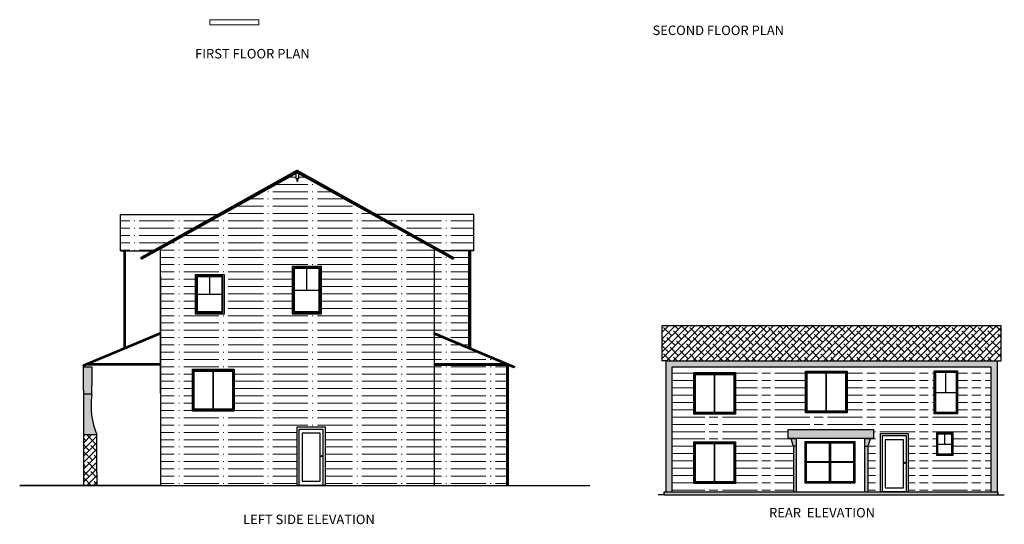
# Model space of a CAD drawing. Units: inches. Extents: x 1838 to 3464, y 573 to 2547.
# Tile 1 of 6: x 2047 to 3464, y 573 to 1299. Entities that reach past the tile are written whole.
import ezdxf

# ---------------------------------------------------------------- set-up
doc = ezdxf.new("R2010")
doc.units = ezdxf.units.IN
for name, color, linetype, lineweight in [('A-ANNO-TEXT', 7, 'Continuous', 18), ('A-DOOR', 4, 'Continuous', 25), ('A-ELEV', 7, 'Continuous', 25), ('A-ELEV-PATT', 252, 'Continuous', 13), ('A-FURN', 8, 'Continuous', 18), ('A-GLAZ', 3, 'Continuous', 25)]:
    doc.layers.add(name, color=color, linetype=linetype, lineweight=lineweight)
doc.styles.get("Standard").update_dxf_attribs({"font": 'arial.ttf'})

# ---------------------------------------------------------------- blocks, each defined once
blk = doc.blocks.new('*U56')
for p, q in [((1.5, 1.5), (1.5, 58.5)), ((1.5, 58.5), (30, 58.5)), ((30, 1.5), (30, 58.5)), ((30, 58.5), (58.5, 58.5)), ((58.5, 58.5), (58.5, 1.5)), ((30, 1.5), (1.5, 1.5)), ((58.5, 1.5), (30, 1.5))]:
    blk.add_line(p, q)
blk.add_lwpolyline([(0, 0), (0, 60), (60, 60), (60, 0)], close=True)
for points in [[(29, 57.5), (29, 2.5), (2.5, 2.5), (2.5, 57.5), (29, 57.5)], [(30, 57.5), (57.5, 57.5), (57.5, 2.5), (30, 2.5)]]:
    blk.add_lwpolyline(points)
blk = doc.blocks.new('*U62')
blk.add_lwpolyline([(3.1, 0), (0.1, 0), (0.1, 84), (40.1, 84), (40.1, 0), (37.1, 0)])
for points in [[(37.1, 81), (37.1, 0), (3.1, 0), (3.1, 81)], [(33.1, 6), (33.1, 75), (7.1, 75), (7.1, 6)]]:
    blk.add_lwpolyline(points, close=True)
blk.add_circle((35.1, 42), 1)

msp = doc.modelspace()

# ---------------------------------------------------------------- hatches: boundary and pattern name
at = {"layer": 'A-ELEV-PATT'}
h = msp.add_hatch(dxfattribs=at)
h.set_pattern_fill('ACAD_ISO04W100', color=256, scale=2.1)
h.set_pattern_definition([(0, (105.552, 127.841), (0, 10.5), [50.4, -6.3, 1.05, -6.3])])
h.paths.add_polyline_path([(2643.45, 925.32), (2643.45, 969.53), (2249.61, 969.53), (2249.61, 932.33), (2249.61, 761.58), (2249.61, 629.13), (2643.45, 629.13)])
h.paths.add_polyline_path([(2295.81, 736.13), (2295.81, 796.13), (2355.81, 796.13), (2355.81, 736.13)], flags=16)
h.paths.add_polyline_path([(2297.31, 737.63), (2297.31, 794.63), (2325.81, 794.63), (2354.31, 794.63), (2354.31, 737.63), (2325.81, 737.63)], flags=0)
h.paths.add_polyline_path([(2298.31, 738.63), (2298.31, 793.63), (2324.81, 793.63), (2324.81, 738.63)], flags=0)
h.paths.add_polyline_path([(2325.81, 793.63), (2353.31, 793.63), (2353.31, 738.63), (2325.81, 738.63)], flags=0)
h.paths.add_polyline_path([(2446.48, 713.14), (2486.48, 713.14), (2486.48, 629.14), (2483.48, 629.14), (2449.48, 629.14), (2446.48, 629.14)], flags=16)
h.paths.add_polyline_path([(2299.61, 876.16), (2299.61, 932.25), (2341.65, 932.25), (2341.65, 876.16)], flags=16)
h.paths.add_polyline_path([(2301.61, 878.16), (2301.61, 930.25), (2339.65, 930.25), (2339.65, 878.16)], flags=0)
h.paths.add_polyline_path([(2453.48, 704.12), (2479.48, 704.12), (2479.48, 635.14), (2453.48, 635.14)], flags=0)
h.paths.add_polyline_path([(2302.61, 879.16), (2302.61, 929.25), (2338.65, 929.25), (2338.65, 879.16)], flags=0)
h.paths.add_polyline_path([(2482.48, 671.14, -1), (2480.48, 671.14, -1)], flags=0)
h.paths.add_polyline_path([(2439.19, 876.16), (2439.19, 944.25), (2481.23, 944.25), (2481.23, 876.16)], flags=16)
h.paths.add_polyline_path([(2441.19, 878.16), (2441.19, 942.25), (2479.23, 942.25), (2479.23, 878.16)], flags=0)
h.paths.add_polyline_path([(2442.19, 879.16), (2442.19, 941.25), (2478.23, 941.25), (2478.23, 879.16)], flags=0)
h.paths.add_polyline_path([(2747.75, 802.06), (2643.45, 802.06), (2643.45, 629.13), (2747.75, 629.13)])
h.paths.add_polyline_path([(2693.56, 966.65), (2654.78, 966.65), (2671.74, 957.2), (2670.28, 954.58), (2643.45, 969.53), (2643.45, 925.32), (2643.45, 849.13), (2644.23, 848.8), (2693.56, 827.96)])
h.paths.add_polyline_path([(2643.45, 846.95), (2643.45, 804.06), (2745.02, 804.06)])
h.paths.add_polyline_path([(2700.73, 1019.23), (2560.36, 1019.23), (2654.78, 966.65), (2693.56, 966.65), (2700.73, 966.65)])
h.paths.add_polyline_path([(2332.7, 1019.23), (2192.33, 1019.23), (2192.33, 966.65), (2238.27, 966.65)])
h.paths.add_polyline_path([(2448.12, 1078.31), (2448.12, 1077.95), (2448.12, 1070.13), (2447.07, 1070.13), (2447.07, 1066.43), (2446.14, 1066.43), (2446.14, 1070.13), (2445.07, 1070.13), (2445.07, 1078.38), (2249.61, 969.53), (2643.45, 969.53)])
h = msp.add_hatch(color=256, dxfattribs=at)
h.dxf.hatch_style = 1
h.paths.add_polyline_path([(2249.61, 846.95), (2249.61, 848.04), (2249.22, 847.88), (2138.23, 801), (2138.62, 800.08)])
h.paths.add_polyline_path([(2249.22, 847.88), (2249.61, 848.04), (2249.61, 849.13), (2248.83, 848.8), (2137.84, 801.92), (2138.23, 801)])
h.paths.add_polyline_path([(2249.61, 803.06), (2145.67, 803.06), (2143.3, 802.06), (2249.61, 802.06)], flags=17)
h.paths.add_polyline_path([(2249.61, 804.06), (2148.04, 804.06), (2145.67, 803.06), (2249.61, 803.06)], flags=17)
h.paths.add_polyline_path([(2199.5, 966.65), (2198.5, 966.65), (2198.5, 827.54), (2199.5, 827.96)])
h = msp.add_hatch(color=256, dxfattribs=at)
h.dxf.hatch_style = 1
h.paths.add_polyline_path([(2198.5, 966.65), (2197.5, 966.65), (2197.51, 827.12), (2198.5, 827.54)])
h = msp.add_hatch(color=256, dxfattribs=at)
h.dxf.hatch_style = 1
h.paths.add_polyline_path([(2695.56, 966.65), (2694.56, 966.65), (2694.56, 950.51), (2694.56, 827.54), (2695.56, 827.54)])
h.paths.add_polyline_path([(2749.75, 802.06), (2748.75, 802.06), (2748.75, 629.13), (2749.75, 629.13)])
h.paths.add_polyline_path([(2748.75, 802.06), (2747.75, 802.06), (2747.75, 629.13), (2748.75, 629.13)])
h.paths.add_polyline_path([(2643.84, 847.88), (2643.45, 848.04), (2643.45, 846.95), (2757.65, 798.72), (2758.55, 799.43)])
h.paths.add_polyline_path([(2745.02, 803.06), (2643.45, 803.06), (2643.45, 802.06), (2745.02, 802.06)], flags=17)
h.paths.add_polyline_path([(2745.02, 804.06), (2643.45, 804.06), (2643.45, 803.06), (2745.02, 803.06)], flags=17)
h.paths.add_polyline_path([(2747.39, 803.06), (2745.02, 803.06), (2745.02, 802.06), (2749.75, 802.06)], flags=17)
h.paths.add_polyline_path([(2745.02, 804.06), (2745.02, 803.06), (2747.39, 803.06)], flags=17)
h.paths.add_polyline_path([(2693.56, 827.96), (2694.56, 827.54), (2694.56, 966.65), (2693.56, 966.65)])
h = msp.add_hatch(dxfattribs=at)
h.set_pattern_fill('ANSI38', color=256, scale=2.1)
h.set_pattern_definition([(45, (-41.478, 118.373), (-4.714634, 4.714634), []), (135, (-41.478, 118.373), (-14.143903, 4.714634), [16.66875, -10.00125])])
h.paths.add_polyline_path([(2971.14, 858.86), (2971.14, 808.58), (2977.14, 808.58), (3453.37, 808.58), (3459.37, 808.58), (3459.37, 858.86)])
h = msp.add_hatch(color=256, dxfattribs=at)
h.dxf.hatch_style = 1
h.paths.add_polyline_path([(2986.14, 799.58), (3444.37, 799.58), (3444.37, 619.58), (3453.37, 619.58), (3453.37, 808.58), (2977.14, 808.58), (2977.14, 739.58), (2977.14, 619.58), (2986.14, 619.58), (2986.14, 739.58)])
h.paths.add_polyline_path([(3454.38, 619.58), (2974.38, 619.58), (2974.38, 615.58), (3454.38, 615.58)])
h.paths.add_polyline_path([(3164.95, 685.75), (3160.45, 685.75), (3160.45, 619.58), (3164.95, 619.58)], flags=17)
h.paths.add_polyline_path([(3267.64, 685.75), (3263.14, 685.75), (3263.14, 619.58), (3267.64, 619.58)], flags=17)
h.paths.add_polyline_path([(3271.49, 696.79), (3263.14, 696.79), (3263.14, 685.75), (3267.64, 685.75, -0.0025316)], flags=17)
h.paths.add_polyline_path([(3164.95, 696.79), (3156.6, 696.79, -0.0025316), (3160.45, 685.75), (3164.95, 685.75)], flags=17)
h.paths.add_polyline_path([(3275.43, 709.65), (3152.67, 709.65), (3152.67, 696.79), (3275.43, 696.79)], flags=17)
h = msp.add_hatch(color=256, dxfattribs=at)
h.dxf.hatch_style = 1
h.paths.add_polyline_path([(2150.81, 759.27), (2150.81, 760.91), (2138.74, 760.91), (2138.74, 701.7), (2158.07, 701.7, -0.1313074)])
h.paths.add_polyline_path([(2150.81, 799.8), (2138.74, 799.8), (2138.74, 766.1), (2138.74, 760.91), (2150.81, 760.91), (2150.81, 772.84)])
h = msp.add_hatch(dxfattribs=at)
h.set_pattern_fill('ACAD_ISO08W100', color=256, scale=2.1)
h.set_pattern_definition([(0, (-41.478, 118.373), (0, 10.5), [50.4, -6.3, 12.6, -6.3])])
h.paths.add_polyline_path([(3444.37, 799.58), (2986.14, 799.58), (2986.14, 739.58), (2986.14, 619.58), (3160.45, 619.58), (3160.45, 685.75, 0.0025316), (3156.6, 696.79), (3152.67, 696.79), (3152.67, 709.65), (3275.43, 709.65), (3275.43, 696.79), (3271.49, 696.79, 0.0025316), (3267.64, 685.75), (3267.64, 619.58), (3444.37, 619.58)])
h.paths.add_polyline_path([(3177.89, 793.35), (3237.89, 793.35), (3237.89, 733.35), (3177.89, 733.35)], flags=16)
h.paths.add_polyline_path([(3179.39, 791.85), (3207.89, 791.85), (3236.39, 791.85), (3236.39, 734.85), (3207.89, 734.85), (3179.39, 734.85)], flags=0)
h.paths.add_polyline_path([(3180.39, 790.85), (3206.89, 790.85), (3206.89, 735.85), (3180.39, 735.85)], flags=0)
h.paths.add_polyline_path([(3207.89, 790.85), (3235.39, 790.85), (3235.39, 735.85), (3207.89, 735.85)], flags=0)
h.paths.add_polyline_path([(3077.17, 731.39), (3017.17, 731.39), (3017.17, 791.39), (3077.17, 791.39)], flags=16)
h.paths.add_polyline_path([(3075.67, 732.89), (3047.17, 732.89), (3018.67, 732.89), (3018.67, 789.89), (3047.17, 789.89), (3075.67, 789.89)], flags=0)
h.paths.add_polyline_path([(3074.67, 733.89), (3047.17, 733.89), (3047.17, 788.89), (3074.67, 788.89)], flags=0)
h.paths.add_polyline_path([(3046.17, 733.89), (3019.67, 733.89), (3019.67, 788.89), (3046.17, 788.89)], flags=0)
h.paths.add_polyline_path([(3077.17, 691.65), (3077.17, 631.65), (3017.17, 631.65), (3017.17, 691.65)], flags=16)
h.paths.add_polyline_path([(3075.67, 690.15), (3075.67, 633.15), (3047.17, 633.15), (3018.67, 633.15), (3018.67, 690.15), (3047.17, 690.15)], flags=0)
h.paths.add_polyline_path([(3074.67, 689.15), (3074.67, 634.15), (3047.17, 634.15), (3047.17, 689.15)], flags=0)
h.paths.add_polyline_path([(3046.17, 634.15), (3019.67, 634.15), (3019.67, 689.15), (3046.17, 689.15)], flags=0)
h.paths.add_polyline_path([(3285.63, 703.67), (3325.63, 703.67), (3325.63, 619.67), (3322.63, 619.67), (3288.63, 619.67), (3285.63, 619.67)], flags=16)
h.paths.add_polyline_path([(3292.63, 694.65), (3318.63, 694.65), (3318.63, 625.67), (3292.63, 625.67)], flags=0)
h.paths.add_polyline_path([(3321.63, 661.67, -1), (3319.63, 661.67, -1)], flags=0)
h.paths.add_polyline_path([(3362.62, 793.52), (3397.19, 793.52), (3397.19, 732.39), (3362.62, 732.39)], flags=16)
h.paths.add_polyline_path([(3363.62, 792.52), (3396.19, 792.52), (3396.19, 733.39), (3363.62, 733.39)], flags=0)
h.paths.add_polyline_path([(3364.62, 791.52), (3395.19, 791.52), (3395.19, 734.39), (3364.62, 734.39)], flags=0)
h.paths.add_polyline_path([(3366.2, 704.57), (3390.2, 704.57), (3390.2, 672.56), (3366.2, 672.56)], flags=16)
h.paths.add_polyline_path([(3367.34, 703.43), (3389.06, 703.43), (3389.06, 673.7), (3367.34, 673.7)], flags=0)
h.paths.add_polyline_path([(3367.91, 702.86), (3388.48, 702.86), (3388.48, 674.27), (3367.91, 674.27)], flags=0)
h = msp.add_hatch(dxfattribs=at)
h.set_pattern_fill('ANSI38', color=256, scale=2.1)
h.set_pattern_definition([(45, (105.5516, 127.841), (-4.714634, 4.714634), []), (135, (105.5516, 127.841), (-14.143903, 4.714634), [16.66875, -10.00125])])
h.paths.add_polyline_path([(2138.74, 647.13), (2138.74, 629.13), (2158.07, 629.13), (2158.07, 647.13), (2158.07, 701.7), (2138.74, 701.7)])

# ---------------------------------------------------------------- linework, layer by layer
at = {"layer": 'A-ELEV'}
for p, q in [((2446.53, 1082.63), (2221.32, 957.2)), ((2221.32, 957.2), (2446.53, 1082.63)), ((2446.53, 1081.48), (2221.81, 956.33)), ((2446.53, 1080.34), (2222.29, 955.46)), ((2446.53, 1079.19), (2222.78, 954.58)), ((2446.53, 1079.19), (2222.78, 954.58)), ((2446.53, 1079.19), (2249.61, 969.53)), ((2249.61, 969.53), (2446.53, 1079.19)), ((2445.07, 1077.95), (2445.07, 1078.38)), ((2446.53, 1082.63), (2671.74, 957.2)), ((2446.53, 1082.63), (2671.74, 957.2)), ((2446.53, 1081.48), (2671.25, 956.33)), ((2446.53, 1080.34), (2670.77, 955.46)), ((2446.53, 1079.19), (2670.28, 954.58)), ((2670.28, 954.58), (2446.53, 1079.19)), ((2448.12, 1077.95), (2448.12, 1078.34)), ((2192.33, 966.65), (2192.33, 1019.23)), ((2192.33, 1019.23), (2332.7, 1019.23)), ((2700.73, 1019.23), (2560.36, 1019.23)), ((2700.73, 966.65), (2700.73, 1019.23)), ((2192.33, 966.65), (2238.27, 966.65)), ((2197.51, 827.12), (2197.5, 966.65)), ((2198.5, 827.54), (2198.5, 966.65)), ((2199.5, 827.54), (2199.5, 966.65)), ((2249.61, 932.33), (2249.61, 969.53)), ((2643.45, 969.53), (2643.45, 925.32)), ((2700.73, 966.65), (2654.78, 966.65)), ((2693.56, 827.96), (2693.56, 966.65)), ((2694.56, 827.54), (2694.56, 966.65)), ((2694.56, 950.51), (2694.56, 966.65)), ((2695.56, 827.54), (2695.56, 966.65)), ((2221.32, 957.2), (2222.78, 954.58)), ((2222.78, 954.58), (2221.32, 957.2)), ((2222.78, 954.58), (2221.32, 957.2)), ((2670.28, 954.58), (2671.74, 957.2)), ((2671.74, 957.2), (2670.28, 954.58)), ((2249.61, 761.58), (2249.61, 932.33)), ((2249.61, 930.1), (2249.61, 629.13)), ((2643.45, 925.32), (2643.45, 629.13)), ((3459.37, 858.86), (2971.14, 858.86)), ((2971.14, 858.86), (2971.14, 808.58)), ((3459.37, 808.58), (3459.37, 858.86)), ((2248.83, 848.8), (2137.84, 801.92)), ((2249.22, 847.88), (2138.23, 801)), ((2249.61, 846.95), (2138.62, 800.08)), ((2248.83, 848.8), (2249.61, 849.13)), ((2249.22, 847.88), (2249.61, 848.04)), ((2644.23, 848.8), (2643.45, 849.13)), ((2643.45, 846.95), (2643.45, 849.13)), ((2643.45, 849.13), (2759.45, 800.13)), ((2643.84, 847.88), (2643.45, 848.04)), ((2643.45, 846.95), (2757.65, 798.72)), ((2757.65, 798.72), (2643.45, 846.95)), ((2643.84, 847.88), (2758.55, 799.43)), ((2644.23, 848.8), (2759.45, 800.13)), ((2693.56, 827.96), (2694.56, 827.54)), ((2977.14, 808.58), (2971.14, 808.58)), ((2977.14, 739.58), (2977.14, 808.58)), ((2977.14, 808.58), (3453.37, 808.58)), ((3453.37, 808.58), (3453.37, 619.58)), ((3453.37, 808.58), (3459.37, 808.58)), ((2137.84, 801.92), (2138.62, 800.08)), ((2138.74, 766.1), (2138.74, 799.8)), ((2138.74, 799.8), (2150.81, 799.8)), ((2249.61, 802.06), (2143.3, 802.06)), ((2249.61, 803.06), (2145.67, 803.06)), ((2249.61, 804.06), (2148.04, 804.06)), ((2150.81, 799.8), (2150.81, 772.84)), ((2745.02, 804.06), (2643.45, 804.06)), ((2747.39, 803.06), (2643.45, 803.06)), ((2749.75, 802.06), (2643.45, 802.06)), ((2749.75, 802.06), (2745.02, 804.06)), ((2745.02, 802.06), (2749.75, 802.06)), ((2747.75, 802.06), (2747.75, 629.13)), ((2748.75, 802.06), (2748.75, 629.13)), ((2749.75, 802.06), (2749.75, 629.13)), ((2757.65, 798.72), (2759.45, 800.13)), ((2759.45, 800.13), (2757.65, 798.72)), ((2986.14, 739.58), (2986.14, 799.58)), ((2986.14, 799.58), (3444.37, 799.58)), ((3444.37, 799.58), (3444.37, 619.58)), ((2138.74, 766.1), (2138.74, 647.13)), ((2150.81, 759.27), (2150.81, 772.84)), ((2138.74, 760.91), (2151.05, 760.91)), ((2977.14, 619.58), (2977.14, 739.58)), ((2986.14, 619.58), (2986.14, 739.58)), ((2158.07, 701.7), (2138.74, 701.7)), ((2158.07, 647.13), (2158.07, 701.7)), ((3152.67, 696.79), (3164.95, 696.79)), ((3164.95, 685.75), (3164.95, 696.79)), ((3263.14, 685.75), (3263.14, 696.79)), ((3263.14, 696.79), (3275.42, 696.79)), ((3164.95, 685.75), (3160.45, 685.75)), ((3160.45, 685.75), (3160.45, 619.58)), ((3164.95, 619.58), (3164.95, 685.75)), ((3263.14, 619.58), (3263.14, 685.75)), ((3263.14, 685.75), (3267.64, 685.75)), ((3267.64, 685.75), (3267.64, 619.58)), ((2138.74, 647.13), (2138.74, 629.13)), ((2158.07, 647.13), (2158.07, 629.13)), ((2249.61, 629.13), (2047.13, 629.13)), ((2047.13, 629.13), (2867.27, 629.13)), ((2249.61, 629.13), (2643.45, 629.13)), ((2974.38, 615.58), (2965.87, 615.58)), ((2974.38, 619.58), (3454.38, 619.58)), ((2974.38, 615.58), (2974.38, 619.58)), ((2974.38, 619.58), (2974.38, 615.58)), ((2974.38, 615.58), (3454.38, 615.58)), ((3454.38, 615.58), (3454.38, 619.58)), ((3454.38, 619.58), (3454.38, 615.58)), ((3454.38, 615.58), (3463.82, 615.58))]:
    msp.add_line(p, q, dxfattribs=at)
for points in [[(2448.12, 1077.95), (2448.12, 1070.13), (2445.07, 1070.13), (2445.07, 1077.95)], [(2693.56, 827.96), (2693.56, 966.65), (2695.56, 966.65), (2695.56, 827.54), (2694.56, 827.54)]]:
    msp.add_lwpolyline(points, dxfattribs=at)
for points in [[(2446.14, 1070.13), (2447.07, 1070.13), (2447.07, 1066.43), (2446.14, 1066.43)], [(2197.5, 966.65), (2198.5, 966.65), (2198.5, 827.09), (2197.5, 827.09)], [(2643.45, 802.06), (2745.02, 802.06), (2745.02, 804.06), (2643.45, 804.06)], [(2747.75, 629.13), (2748.75, 629.13), (2748.75, 802.06), (2747.75, 802.06)], [(2748.75, 802.06), (2749.75, 802.06), (2749.75, 629.13), (2748.75, 629.13)], [(3275.43, 696.79), (3152.67, 696.79), (3152.67, 709.65), (3275.43, 709.65)]]:
    msp.add_lwpolyline(points, close=True, dxfattribs=at)
for centre, radius, start, end in [((2262.15, 744.07), 112.38, 172.22809, 202.15034), ((2067.71, 310.68), 1155.32, 18.94422, 19.52441), ((4360.38, 310.68), 1155.32, 160.47559, 161.05578)]:
    msp.add_arc(centre, radius, start, end, dxfattribs=at)
at = {"layer": 'A-FURN'}
msp.add_lwpolyline([(2320.67, 1299.46), (2391.42, 1299.46), (2391.42, 1292.16), (2320.67, 1292.16)], close=True, dxfattribs=at)
at = {"layer": 'A-GLAZ'}
for p, q in [((2460.21, 910.21), (2460.21, 941.25)), ((2320.63, 904.21), (2320.63, 929.25)), ((2442.19, 910.21), (2478.23, 910.21)), ((2302.61, 904.21), (2338.65, 904.21)), ((3379.91, 762.96), (3379.91, 791.52)), ((3364.62, 762.96), (3395.19, 762.96)), ((3378.2, 688.56), (3378.2, 702.86)), ((3211.96, 692.21), (3211.96, 632.41)), ((3212.96, 692.21), (3212.96, 632.41)), ((3213.96, 692.21), (3213.96, 632.41)), ((3367.91, 688.56), (3388.48, 688.56)), ((3179.1, 663.31), (3246.81, 663.31)), ((3179.1, 662.31), (3246.81, 662.31))]:
    msp.add_line(p, q, dxfattribs=at)
for points in [[(2439.19, 876.16), (2481.23, 876.16), (2481.23, 944.25), (2439.19, 944.25)], [(2441.19, 878.16), (2479.23, 878.16), (2479.23, 942.25), (2441.19, 942.25)], [(2442.19, 879.16), (2478.23, 879.16), (2478.23, 941.25), (2442.19, 941.25)], [(2299.61, 876.16), (2341.65, 876.16), (2341.65, 932.25), (2299.61, 932.25)], [(2301.61, 878.16), (2339.65, 878.16), (2339.65, 930.25), (2301.61, 930.25)], [(2302.61, 879.16), (2338.65, 879.16), (2338.65, 929.25), (2302.61, 929.25)], [(3362.62, 732.39), (3397.19, 732.39), (3397.19, 793.52), (3362.62, 793.52)], [(3363.62, 733.39), (3396.19, 733.39), (3396.19, 792.52), (3363.62, 792.52)], [(3364.62, 734.39), (3395.19, 734.39), (3395.19, 791.52), (3364.62, 791.52)], [(3366.2, 672.56), (3390.2, 672.56), (3390.2, 704.57), (3366.2, 704.57)], [(3367.34, 673.7), (3389.06, 673.7), (3389.06, 703.43), (3367.34, 703.43)], [(3367.91, 674.27), (3388.48, 674.27), (3388.48, 702.86), (3367.91, 702.86)], [(3177.1, 692.21), (3248.81, 692.21), (3248.81, 632.41), (3177.1, 632.41)], [(3178.1, 691.21), (3247.81, 691.21), (3247.81, 633.41), (3178.1, 633.41)], [(3179.1, 690.21), (3246.81, 690.21), (3246.81, 634.41), (3179.1, 634.41)]]:
    msp.add_lwpolyline(points, close=True, dxfattribs=at)

# ---------------------------------------------------------------- block references
at = {"layer": 'A-DOOR'}
for p in [(2446.35, 629.13), (3285.51, 619.66)]:
    msp.add_blockref('*U62', p, dxfattribs=at)
at = {"layer": 'A-GLAZ'}
for p in [(2295.81, 736.13), (3177.89, 733.35), (3017.17, 731.39), (3017.17, 631.65)]:
    msp.add_blockref('*U56', p, dxfattribs=at)

# ---------------------------------------------------------------- texts
at = {"layer": 'A-ANNO-TEXT', "char_height": 13.6813, "attachment_point": 1}
for s, width, insert in [('SECOND FLOOR PLAN', 275.9918, (2957.63, 1290.99)), ('FIRST FLOOR PLAN', 191.1523, (2299.42, 1257.35)), ('REAR  ELEVATION', 275.9918, (3125.3, 596.67)), ('LEFT SIDE ELEVATION', 275.9918, (2368.52, 586.94))]:
    msp.add_mtext_dynamic_manual_height_columns(s, width=width, gutter_width=68.41, heights=[0], dxfattribs=dict(at, insert=insert))

doc.saveas('drawing.dxf')
